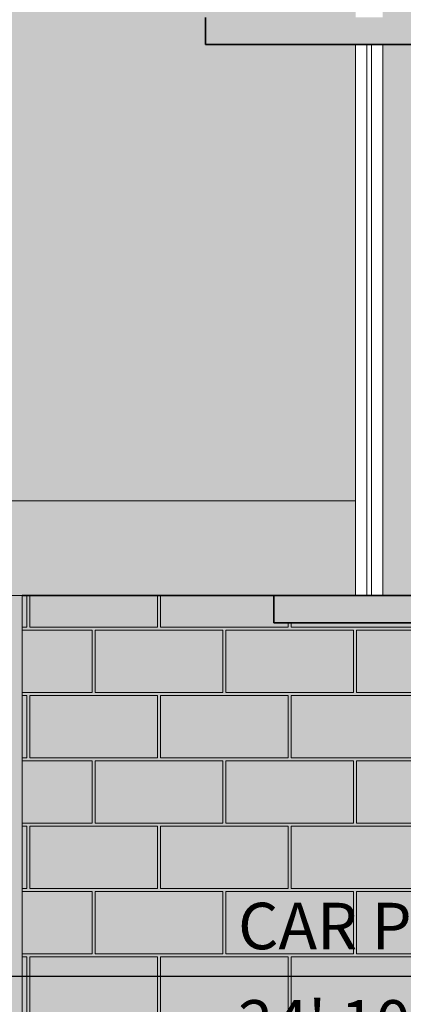
# Model space of a CAD drawing. Units: inches. Extents: x 1704 to 6393, y -157 to 1172.
# Tile 19 of 122: x 1975 to 2087, y 82 to 372. Entities that reach past the tile are written whole.
import ezdxf

# ---------------------------------------------------------------- set-up
doc = ezdxf.new("R2010")
doc.units = ezdxf.units.IN
doc.header["$MEASUREMENT"] = 0
for name, color, linetype, lineweight in [('A-ANNO-DIMS', 7, 'Continuous', 13), ('A-AREA-IDEN', 7, 'Continuous', 18), ('A-WALL-PATT', 7, 'Continuous', 13), ('GLASS PANEL FASADE', 4, 'Continuous', 18), ('L-HRDS', 8, 'Continuous', 18), ('L-PVMT-PATT', 8, 'Continuous', 13), ('WALLS', 7, 'Continuous', 35)]:
    doc.layers.add(name, color=color, linetype=linetype, lineweight=lineweight)
for name, color, linetype, lineweight, true_color in [('A-FLOR-PATT', 7, 'Continuous', 13, 0xf2f2f2), ('L-HRDS-PATT', 9, 'Continuous', 13, 0xc5c1ba), ('L-PLNT-PATT', 253, 'Continuous', 13, 0x9abc8f)]:
    doc.layers.add(name, color=color, linetype=linetype, lineweight=lineweight, true_color=true_color)
doc.styles.get("Standard").update_dxf_attribs({"font": 'arial.ttf'})
doc.dimstyles.get("Standard").update_dxf_attribs({"dimtxt": 6, "dimasz": 2, "dimexe": 0.18, "dimexo": 0.0625, "dimgap": 0.09, "dimtad": 0, "dimtih": 1, "dimtoh": 1, "dimdec": 1, "dimzin": 0, "dimdsep": 46, "dimlunit": 3, "dimtxsty": 'Standard', "dimblk": 'ARCHTICK', "dimcen": 0.09, "dimadec": 0, "dimazin": 0, "dimtfac": 1, "dimtdec": 1, "dimtofl": 0, "dimtmove": 0, "dimatfit": 3, "dimfxl": 1, "dimtolj": 1, "dimtzin": 0, "dimarcsym": 0})

# ---------------------------------------------------------------- blocks, each defined once
blk = doc.blocks.new('GLAZ-PANEL-162')
for p, q in [((3.3, 0), (3.3, 162)), ((4.7, 0), (4.7, 162))]:
    blk.add_line(p, q)
blk.add_lwpolyline([(8, 0), (0, 0), (0, 162), (8, 162)], close=True)
blk = doc.blocks.new('_ArchTick')
at = {"color": 0, "linetype": 'ByBlock', "const_width": 0.15}
blk.add_lwpolyline([(-0.5, -0.5), (0.5, 0.5)], dxfattribs=at)
blk = doc.blocks.new('*D93')
at = {"layer": 'A-ANNO-DIMS', "color": 0, "lineweight": -2, "transparency": 16777216}
for p, q in [((2605.29, 895.21), (1829.7, 895.21)), ((1829.88, 895.21), (1829.88, 495.87)), ((1829.88, 90.21), (1829.88, 489.56)), ((2605.29, 90.21), (1829.7, 90.21))]:
    blk.add_line(p, q, dxfattribs=at)
at = {"layer": 'Defpoints', "color": 0, "lineweight": -3, "transparency": 16777216}
for p in [(2605.35, 895.21), (1829.88, 90.21), (2605.35, 90.21)]:
    blk.add_point(p, dxfattribs=at)
at = {"layer": 'A-ANNO-DIMS', "color": 0, "lineweight": -2, "transparency": 16777216, "xscale": 2, "yscale": 2, "zscale": 2}
for p, rotation in [((1829.88, 895.21), 90), ((1829.88, 90.21), 270)]:
    blk.add_blockref('_ArchTick', p, dxfattribs=dict(at, rotation=rotation))
at = {"layer": 'A-ANNO-DIMS', "color": 0, "transparency": 16777216, "insert": (1829.88, 492.71), "char_height": 6, "attachment_point": 5}
blk.add_mtext('\\A1;805', dxfattribs=at)

msp = doc.modelspace()

# ---------------------------------------------------------------- hatches: boundary and pattern name
at = {"layer": 'A-FLOR-PATT', "transparency": 33554528}
h = msp.add_hatch(color=256, dxfattribs=at)
h.dxf.hatch_style = 1
h.paths.add_polyline_path([(2273.349, 538.213), (2081.349, 538.213), (2081.349, 372.213), (2273.349, 372.213)])
h.paths.add_polyline_path([(2189.542, 505.951), (2184.316, 505.951), (2184.316, 505.591), (2169.442, 505.591), (2169.442, 505.951), (2164.216, 505.951, -0.4142136), (2163.814, 506.353), (2163.814, 526.093, -0.4142136), (2164.216, 526.495), (2189.542, 526.495, -0.4142136), (2189.944, 526.093), (2189.944, 506.353, -0.4142136)], flags=16)
h.paths.add_polyline_path([(2200.535, 511.491), (2200.535, 526.191), (2217.621, 526.191), (2217.621, 511.491), (2214.605, 511.491, -0.3946213), (2214.203, 511.116), (2203.952, 511.116, -0.3946213), (2203.551, 511.491)], flags=16)
h.paths.add_polyline_path([(2200.736, 511.692), (2200.736, 525.99), (2203.55, 525.99), (2203.55, 523.838, 0.1045605), (2214.605, 523.838), (2214.605, 525.99), (2217.42, 525.99), (2217.42, 511.692), (2214.605, 511.692), (2214.605, 523.838, -0.1045605), (2203.55, 523.838), (2203.55, 511.692)], flags=0)
h.paths.add_polyline_path([(2203.952, 511.317, -0.4142136), (2203.751, 511.518), (2203.751, 523.591, 0.099912), (2214.404, 523.591), (2214.404, 511.518, -0.4142136), (2214.203, 511.317)], flags=0)
h.paths.add_polyline_path([(2184.084, 516.015, -0.0686795), (2169.674, 516.015), (2169.674, 522.073), (2184.084, 522.073)], flags=0)
h.paths.add_polyline_path([(2183.325, 518.606, -0.0772766), (2170.433, 518.606), (2170.433, 521.123, -0.0235462), (2183.325, 521.123)], flags=0)
h.paths.add_polyline_path([(2135.029, 507.225, -0.1405189), (2135.191, 507.834, -0.0513838), (2135.029, 507.797)], flags=16)
h.paths.add_polyline_path([(2146.318, 498.997, -0.0311848), (2144.279, 499.202, -0.1719602), (2141.865, 499.263, -0.2234326), (2139.482, 499.263, -0.1719602), (2137.068, 499.202, -0.0311848), (2135.029, 498.997, -0.066975), (2135.029, 505.313, -0.0276914), (2136.841, 505.144), (2136.841, 506.777), (2136.576, 506.777), (2136.576, 507.371, 0.039911), (2145.741, 507.448, 0.2546956), (2146.318, 507.225), (2146.318, 507.269, 0.1305786), (2146.156, 507.834, -0.0704067), (2145.953, 507.935, -0.011584), (2145.714, 508.002, -0.2546956), (2145.137, 507.779, -0.2546956), (2145.361, 508.355, -0.0259693), (2145.107, 516.407, -0.0070422), (2144.025, 516.297, -0.1828112), (2142.939, 516.218, -0.2042746), (2142.015, 516.175, -0.1805419), (2139.348, 516.174, -0.0000184), (2139.345, 516.174, -0.2035615), (2138.425, 516.217, -0.0000237), (2138.421, 516.217, -0.1818152), (2137.34, 516.296, -0.0071635), (2136.24, 516.407, 0.007166), (2136.162, 518.63, 0.314303), (2135.854, 518.974, -0.1253469), (2135.537, 518.935, -0.2546956), (2135.76, 519.512, -0.0162662), (2135.67, 519.849, -0.296972), (2135.535, 520.8, -0.227702), (2135.464, 521.698, 0.1283977), (2132.757, 521.718), (2132.757, 525.785, -0.4142136), (2133.331, 526.359), (2148.015, 526.359, -0.4142136), (2148.589, 525.785), (2148.589, 521.718, -0.0118936), (2148.835, 521.65, -0.2546956), (2149.412, 521.873, -0.2546956), (2149.188, 521.296, -0.0417628), (2149.188, 508.355, -0.2546956), (2149.412, 507.779, -0.2546956), (2148.835, 508.002, -0.011584), (2148.596, 507.935, -0.2124435), (2147.949, 507.813, -0.2363999), (2147.423, 507.772, -0.3143526), (2147.126, 507.772, -0.2363999), (2146.6, 507.813, -0.0879275), (2146.318, 507.797), (2146.318, 507.225, -0.2546956), (2145.741, 507.448, -0.0042329), (2144.771, 507.371), (2144.771, 506.777), (2144.506, 506.777), (2144.506, 505.144, -0.0276914), (2146.318, 505.313, -0.066975)], flags=16)
h.paths.add_polyline_path([(2141.865, 505.047, 0.2234326), (2139.482, 505.047, 0.1738145), (2137.043, 505.1), (2137.043, 506.317), (2137.335, 506.317), (2137.335, 505.184, -0.1522072), (2139.482, 505.047, -0.2234326), (2141.865, 505.047, -0.1522072), (2144.011, 505.184), (2144.011, 506.317), (2144.304, 506.317), (2144.304, 505.1, 0.1738145)], flags=0)
h.paths.add_polyline_path([(2145.233, 522.986, 0.0079197), (2144.017, 523.111, 0.1826165), (2142.931, 523.19, 0.2042746), (2142.008, 523.233, 0.1806536), (2139.339, 523.233, 0.2042746), (2138.415, 523.19, 0.1826165), (2137.33, 523.111, 0.0079197), (2136.114, 522.986, 0.1967082), (2135.679, 523.212, 0.047677), (2135.755, 524.004), (2134.638, 521.852), (2134.376, 524.691, -0.2583282), (2135.029, 526.359, -0.0890464), (2135.632, 525.01, -0.1830277), (2145.715, 525.01, -0.0890464), (2146.318, 526.359, -0.2583282), (2146.971, 524.691), (2146.709, 521.852), (2145.592, 524.004, 0.047677), (2145.668, 523.212, 0.1967082)], flags=0)
h.paths.add_polyline_path([(2144.419, 519.027, -0.0368796), (2136.927, 519.027, -0.0368796)], flags=0)
h.paths.add_polyline_path([(2273.349, 629.213), (2213.349, 629.213), (2213.349, 573.213), (2213.349, 545.213), (2273.349, 545.213)])
h.paths.add_polyline_path([(2273.349, 711.213), (2207.349, 711.213), (2207.349, 709.213), (2231.349, 709.213), (2231.349, 707.213), (2207.349, 707.213), (2207.349, 631.213), (2273.349, 631.213)])
h.paths.add_polyline_path([(2273.349, 364.213), (2081.349, 364.213), (2081.349, 202.213), (2225.349, 202.213), (2229.181, 202.213), (2230.482, 202.213), (2268.215, 202.213), (2269.516, 202.213), (2273.349, 202.213)])
h.paths.add_polyline_path([(2203.551, 339.558, 0.3946213), (2203.952, 339.183), (2214.203, 339.183), (2214.203, 339.384), (2203.751, 339.384), (2203.751, 339.558)], flags=16)
h.paths.add_polyline_path([(2203.55, 351.7), (2203.55, 339.759), (2200.535, 339.759), (2200.535, 354.258), (2217.621, 354.258), (2217.621, 339.558), (2214.404, 339.558), (2214.404, 351.659, -0.101837)], flags=16)
h.paths.add_polyline_path([(2214.404, 354.057), (2214.605, 354.057), (2214.605, 354.258), (2214.404, 354.258)], flags=16)
h.paths.add_polyline_path([(2189.542, 334.018), (2184.316, 334.018), (2184.316, 333.658), (2169.442, 333.658), (2169.442, 334.018), (2164.216, 334.018, -0.4142136), (2163.814, 334.42), (2163.814, 354.161, -0.4142136), (2164.216, 354.563), (2189.542, 354.563, -0.4142136), (2189.944, 354.161), (2189.944, 334.42, -0.4142136)], flags=16)
h.paths.add_polyline_path([(2184.084, 344.083, -0.0686795), (2169.674, 344.083), (2169.674, 349.85), (2165.7, 350.14), (2188.058, 350.14), (2184.084, 349.85)], flags=0)
h.paths.add_polyline_path([(2183.325, 346.673, -0.0772766), (2170.433, 346.673), (2170.433, 349.19, -0.0235462), (2183.325, 349.19)], flags=0)
h.paths.add_polyline_path([(2134.638, 349.919), (2134.376, 352.758, -0.2583282), (2135.029, 354.426), (2133.331, 354.426, 0.4142136), (2132.757, 353.852), (2132.757, 349.785, -0.0886664)], flags=16)
h.paths.add_polyline_path([(2136.114, 351.053, -0.0079197), (2137.33, 351.178, -0.1826165), (2138.415, 351.257, -0.2042746), (2139.339, 351.3, -0.1806536), (2142.008, 351.3, -0.2042746), (2142.931, 351.257, -0.1826165), (2144.017, 351.178, -0.0079197), (2145.233, 351.053, -0.1967082), (2145.668, 351.279, -0.047677), (2145.592, 352.071, 0.1133241), (2135.755, 352.071, -0.047677), (2135.679, 351.279, -0.1967082)], flags=16)
h.paths.add_polyline_path([(2145.184, 346.697, 0.0331414), (2145.361, 336.423, 0.2546956), (2145.137, 335.846, 0.3030408), (2145.781, 336.164, 0.2903634), (2146.6, 335.88, 0.2363999), (2147.126, 335.839, -0.280712), (2147.275, 336.69, -0.280712), (2147.423, 335.839, 0.2363999), (2147.949, 335.88, 0.2903634), (2148.768, 336.164, 0.3030408), (2149.412, 335.846, 0.2546956), (2149.188, 336.423, 0.0417628), (2149.188, 349.363, 0.2546956), (2149.412, 349.94, 0.2546956), (2148.835, 349.717, 0.1405058), (2145.883, 349.765, -0.227702), (2145.812, 348.867, -0.296972), (2145.677, 347.916, -0.0162662), (2145.586, 347.579, -0.2546956), (2145.81, 347.002, -0.1253469), (2145.493, 347.041, 0.314303)], flags=16)
h.paths.add_polyline_path([(2135.029, 335.292, -0.1405189), (2135.191, 335.901, -0.1399435), (2134.747, 335.88, -0.2363999), (2134.22, 335.839, -0.3143526), (2133.924, 335.839, -0.280712), (2134.072, 336.69, -0.280712), (2134.22, 335.839, 0.2363999), (2134.747, 335.88, 0.2903634), (2135.566, 336.164, 0.3030408), (2136.209, 335.846, 0.2546956), (2135.985, 336.423, 0.0331414), (2136.162, 346.697, 0.314303), (2135.854, 347.041, -0.1253469), (2135.537, 347.002, -0.2546956), (2135.76, 347.579, -0.0162662), (2135.67, 347.916, -0.296972), (2135.535, 348.867, -0.2999866), (2135.599, 350.01, -0.0330719), (2135.76, 350.7, -0.3502076), (2135.604, 351.492), (2134.638, 349.919), (2135.604, 351.492, 0.3502076), (2135.76, 350.7, 0.0330719), (2135.599, 350.01, 0.2999866), (2135.535, 348.867, 0.296972), (2135.67, 347.916, 0.0279375), (2135.971, 347.698, 0.3576436), (2135.537, 347.002, 0.1253469), (2135.854, 347.041, -0.3555912), (2136.165, 346.637, -0.0329482), (2135.985, 336.423, -0.2546956), (2136.209, 335.846, -0.2546956), (2135.632, 336.069, -0.011584), (2135.393, 336.003, -0.1222327), (2135.029, 335.864)], flags=16)
h.paths.add_polyline_path([(2136.841, 335.42), (2136.783, 335.423), (2136.783, 334.844), (2136.841, 334.471)], flags=16)
h.paths.add_polyline_path([(2146.318, 327.064, -0.0311848), (2144.279, 327.269, -0.1719602), (2141.865, 327.33, -0.2234326), (2139.482, 327.33, -0.1719602), (2137.068, 327.269, -0.0311848), (2135.029, 327.064, -0.066975), (2135.029, 333.38, -0.0311848), (2137.068, 333.175, -0.1719602), (2139.482, 333.114, -0.2234326), (2141.865, 333.114, -0.1522072), (2144.011, 333.251), (2144.011, 334.384), (2144.304, 335.406, 0.0020345), (2144.771, 335.438), (2144.771, 334.844), (2144.506, 333.211, -0.0276914), (2146.318, 333.38, -0.066975)], flags=16)
h.paths.add_polyline_path([(2137.129, 334.384), (2137.335, 334.384), (2137.335, 333.251), (2137.129, 333.195)], flags=16)
h.paths.add_polyline_path([(2144.419, 347.094, -0.0368796), (2136.927, 347.094, -0.0368796)], flags=16)
at = {"layer": 'A-WALL-PATT', "transparency": 33554643}
h = msp.add_hatch(color=256, dxfattribs=at)
h.dxf.hatch_style = 1
h.paths.add_polyline_path([(2167.349, 895.213), (2073.349, 895.213), (2073.349, 887.213), (2081.349, 887.213), (2167.349, 887.213)])
h.paths.add_polyline_path([(2465.349, 895.213), (2273.349, 895.213), (2273.349, 903.213), (2263.349, 903.213), (2263.349, 895.213), (2263.349, 887.213), (2325.349, 887.213), (2325.349, 863.213), (2333.349, 863.213), (2333.349, 887.213), (2465.349, 887.213)])
h.paths.add_polyline_path([(2533.349, 895.213), (2513.349, 895.213), (2513.349, 887.213), (2513.349, 861.213), (2517.349, 861.213), (2517.349, 887.213), (2533.349, 887.213)])
h.paths.add_polyline_path([(2605.349, 895.213), (2581.349, 895.213), (2581.349, 887.213), (2597.349, 887.213), (2597.349, 854.213), (2605.349, 854.213)])
h.paths.add_polyline_path([(2605.349, 752.213), (2629.349, 752.213), (2629.349, 716.213), (2605.349, 716.213), (2605.349, 712.213), (2719.349, 712.213), (2719.349, 716.213), (2631.349, 716.213), (2631.349, 754.213), (2605.349, 754.213), (2605.349, 794.213), (2597.349, 794.213), (2597.349, 787.213), (2517.349, 787.213), (2517.349, 813.213), (2513.349, 813.213), (2513.349, 783.213), (2517.349, 783.213), (2597.349, 783.213), (2597.349, 719.213), (2517.349, 719.213), (2517.349, 753.213), (2513.349, 753.213), (2513.349, 719.213), (2365.349, 719.213), (2365.349, 763.213), (2325.349, 763.213), (2325.349, 755.213), (2357.349, 755.213), (2357.349, 719.213), (2325.349, 719.213), (2325.349, 711.213), (2547.349, 711.213), (2547.349, 615.213), (2449.349, 615.213), (2449.349, 607.213), (2514.349, 607.213), (2514.349, 546.213), (2439.349, 546.213), (2425.349, 546.213), (2425.349, 607.213), (2425.349, 615.213), (2350.349, 615.213), (2350.349, 589.713), (2358.349, 589.713), (2358.349, 610.213), (2420.349, 610.213), (2420.349, 545.213), (2358.349, 545.213), (2358.349, 565.713), (2350.349, 565.713), (2350.349, 538.213), (2469.349, 538.213), (2469.349, 459.213), (2469.349, 372.213), (2423.349, 372.213), (2423.349, 364.213), (2473.349, 364.213), (2473.349, 318.213), (2477.349, 318.213), (2477.349, 364.213), (2547.349, 364.213), (2547.349, 352.213), (2549.349, 352.213), (2549.349, 364.213), (2597.349, 364.213), (2597.349, 328.213), (2549.349, 328.213), (2547.349, 328.213), (2547.349, 326.213), (2549.349, 326.213), (2597.349, 326.213), (2605.349, 326.213), (2605.349, 377.057), (2597.349, 377.057), (2597.349, 372.213), (2477.349, 372.213), (2477.349, 451.213), (2597.349, 451.213), (2605.349, 451.213), (2605.349, 459.213), (2597.349, 459.213), (2477.349, 459.213), (2477.349, 538.213), (2597.349, 538.213), (2597.349, 495.213), (2605.349, 495.213), (2605.349, 512.213), (2631.349, 512.213), (2631.349, 568.213), (2605.349, 568.213), (2605.349, 577.213), (2597.349, 577.213), (2597.349, 542.213), (2518.349, 542.213), (2518.349, 607.213), (2532.349, 607.213), (2605.349, 607.213), (2605.349, 615.213), (2597.349, 615.213), (2551.349, 615.213), (2551.349, 711.213), (2597.349, 711.213), (2597.349, 645.213), (2605.349, 645.213), (2605.349, 712.213), (2605.349, 716.213)])
h.paths.add_polyline_path([(2605.349, 566.213), (2629.349, 566.213), (2629.349, 514.213), (2605.349, 514.213)], flags=16)
h.paths.add_polyline_path([(2381.349, 372.213), (2349.349, 372.213), (2349.349, 202.213), (2337.349, 202.213), (2337.349, 194.213), (2349.349, 194.213), (2349.349, 90.213), (2349.349, 72.213), (2357.349, 72.213), (2357.349, 90.213), (2381.349, 90.213), (2381.349, 98.213), (2357.349, 98.213), (2357.349, 266.213), (2381.349, 266.213), (2381.349, 270.213), (2353.349, 270.213), (2353.349, 364.213), (2381.349, 364.213)])
h.paths.add_polyline_path([(2605.349, 302.213), (2597.349, 302.213), (2597.349, 270.213), (2477.349, 270.213), (2477.349, 294.213), (2473.349, 294.213), (2473.349, 270.213), (2423.349, 270.213), (2423.349, 266.213), (2597.349, 266.213), (2597.349, 218.213), (2605.349, 218.213)])
h.paths.add_polyline_path([(2605.349, 146.213), (2597.349, 146.213), (2597.349, 98.213), (2429.349, 98.213), (2429.349, 90.213), (2597.349, 90.213), (2597.349, 72.213), (2605.349, 72.213), (2605.349, 90.213)])
h.paths.add_polyline_path([(2225.349, 202.213), (2049.349, 202.213), (2049.349, 194.213), (2225.349, 194.213)])
h.paths.add_polyline_path([(2289.349, 202.213), (2277.349, 202.213), (2273.349, 202.213), (2269.516, 202.213), (2269.516, 194.213), (2273.349, 194.213), (2277.349, 194.213), (2289.349, 194.213)])
h.paths.add_polyline_path([(2273.349, 372.213), (2029.19, 372.213), (2029.19, 364.213), (2273.349, 364.213)])
h.paths.add_polyline_path([(2277.349, 545.213), (2213.349, 545.213), (2213.349, 573.213), (2205.349, 573.213), (2177.349, 573.213), (2177.349, 545.213), (2073.349, 545.213), (2073.349, 538.213), (2081.349, 538.213), (2277.349, 538.213)])
h.paths.add_polyline_path([(2181.349, 545.213), (2181.349, 569.213), (2205.349, 569.213), (2205.349, 545.213)], flags=16)
h.paths.add_polyline_path([(2277.349, 719.213), (2081.349, 719.213), (2073.349, 719.213), (2073.349, 711.213), (2154.575, 711.213), (2205.349, 711.213), (2205.349, 687.213), (2205.349, 629.213), (2213.349, 629.213), (2273.349, 629.213), (2273.349, 631.213), (2207.349, 631.213), (2207.349, 707.213), (2231.349, 707.213), (2231.349, 709.213), (2207.349, 709.213), (2207.349, 711.213), (2277.349, 711.213)])
at = {"layer": 'L-HRDS-PATT', "transparency": 33554643}
h = msp.add_hatch(color=256, dxfattribs=at)
h.dxf.hatch_style = 1
h.paths.add_polyline_path([(1955.732, 380.213), (1916.214, 380.213), (1916.214, 325.779), (1955.732, 325.779)])
h.paths.add_polyline_path([(1955.732, 318.405), (1916.214, 318.405), (1916.214, 279.355), (1955.732, 279.355)])
h.paths.add_polyline_path([(1955.732, 270.314), (1916.214, 270.314), (1916.214, 234.313), (1955.732, 234.313)])
h.paths.add_polyline_path([(2073.349, 230.029), (1898.349, 230.029), (1898.349, 202.213), (2073.349, 202.213)])
at = {"layer": 'L-HRDS-PATT', "transparency": 33554646}
h = msp.add_hatch(color=256, dxfattribs=at)
h.dxf.hatch_style = 1
h.paths.add_polyline_path([(2273.349, 194.213), (2269.516, 194.213), (2268.215, 194.213), (2230.482, 194.213), (2229.181, 194.213), (2225.349, 194.213), (2049.349, 194.213), (2049.349, 202.213), (1975.349, 202.213), (1975.349, -3.787), (2273.349, -3.787)])
at = {"layer": 'L-PLNT-PATT', "transparency": 33554643}
h = msp.add_hatch(color=256, dxfattribs=at)
h.dxf.hatch_style = 1
h.paths.add_polyline_path([(2073.349, 364.213), (2029.19, 364.213), (2029.19, 372.213), (2073.349, 372.213), (2073.349, 380.213), (1955.732, 380.213), (1955.732, 325.779), (1916.214, 325.779), (1916.214, 380.213), (1898.349, 380.213), (1898.349, 230.029), (2073.349, 230.029)])
h.paths.add_polyline_path([(1955.732, 279.355), (1916.214, 279.355), (1916.214, 318.405), (1955.732, 318.405)], flags=16)
h.paths.add_polyline_path([(1955.732, 270.314), (1955.732, 234.313), (1916.214, 234.313), (1916.214, 270.314)], flags=16)
h = msp.add_hatch(color=256, dxfattribs=at)
h.dxf.hatch_style = 1
h.paths.add_polyline_path([(1975.349, 202.213), (1898.349, 202.213), (1898.349, -3.787), (1975.349, -3.787)])
at = {"layer": 'L-PVMT-PATT', "transparency": 33554643}
h = msp.add_hatch(dxfattribs=at)
h.set_pattern_fill('AR-B816C', color=256, scale=2.4)
h.paths.add_polyline_path([(2273.349, 194.213), (2269.516, 194.213), (2268.215, 194.213), (2230.482, 194.213), (2229.181, 194.213), (2225.349, 194.213), (2049.349, 194.213), (2049.349, 202.213), (1975.349, 202.213), (1975.349, -3.787), (2273.349, -3.787)])

# ---------------------------------------------------------------- linework, layer by layer
at = {"layer": 'L-HRDS'}
for q in [(1898.349, 202.213), (1975.349, -3.787)]:
    msp.add_line((1975.349, 202.213), q, dxfattribs=at)
msp.add_lwpolyline([(1898.349, 202.213), (2073.349, 202.213), (2073.349, 230.029), (1898.349, 230.029)], close=True, dxfattribs=at)
at = {"layer": 'WALLS'}
for p, q in [((2029.19, 364.213), (2029.19, 372.213)), ((2277.349, 364.213), (2029.19, 364.213)), ((2225.349, 202.213), (1975.349, 202.213)), ((2049.349, 202.213), (2049.349, 194.213)), ((2225.349, 194.213), (2049.349, 194.213))]:
    msp.add_line(p, q, dxfattribs=at)

# ---------------------------------------------------------------- block references
at = {"layer": 'GLASS PANEL FASADE'}
msp.add_blockref('GLAZ-PANEL-162', (2073.349, 202.213), dxfattribs=at)

# ---------------------------------------------------------------- texts
at = {"layer": 'A-ANNO-DIMS'}
msp.add_text('24\' 10" X 16\' 6"', height=13.6672, dxfattribs=at).set_placement((2038.807, 69.622))
at = {"layer": 'A-AREA-IDEN'}
msp.add_text('CAR PORCH', height=13.6672, dxfattribs=at).set_placement((2038.807, 98.244))

# ---------------------------------------------------------------- dimensions: what is measured, and where the dimension line sits
at = {"layer": 'A-ANNO-DIMS'}
dim = msp.add_linear_dim(base=(1829.878, 90.213), p1=(2605.349, 895.213), p2=(2605.349, 90.213), angle=90, dimstyle='Standard', override={"dimdec": 0, "dimlfac": 1, "dimrnd": 0, "dimzin": 0, "dimdsep": 46, "dimlunit": 2}, dxfattribs=at)
dim.commit()
dim.dimension.update_dxf_attribs({"geometry": '*D93', "text_midpoint": (1829.878, 492.713)})

doc.saveas('drawing.dxf')
